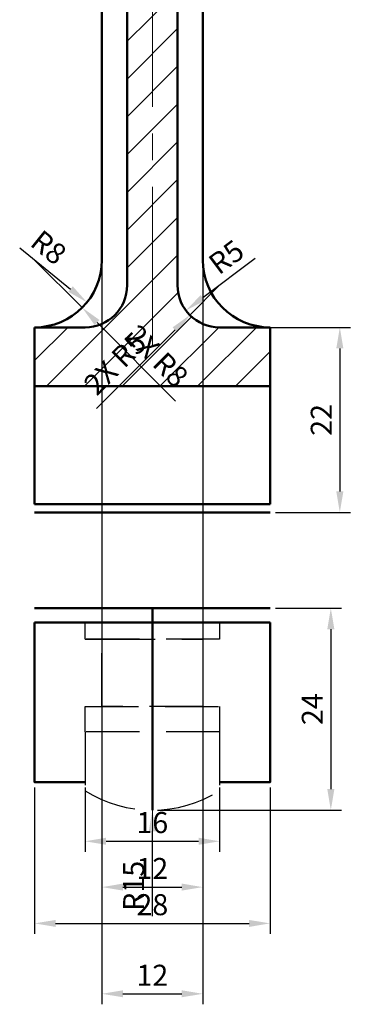
# Model space of a CAD drawing. Units: millimetres. Extents: x 2995 to 3180, y 2734 to 2968.
# Tile 2 of 3: x 3141 to 3180, y 2734 to 2851. Entities that reach past the tile are written whole.
import ezdxf

# ---------------------------------------------------------------- set-up
doc = ezdxf.new("R2010")
doc.units = ezdxf.units.MM
doc.linetypes.add('CENTER2', pattern=[28.575, 19.05, -3.175, 3.175, -3.175])
doc.linetypes.add('HIDDEN', pattern=[9.525, 6.35, -3.175])
for name, color, linetype, lineweight in [('M-CNTR', 1, 'CENTER2', 18), ('M-DIMS', 2, 'Continuous', 25), ('M-HATC', 8, 'Continuous', 18), ('M-HIDN', 4, 'HIDDEN', 25), ('M-OUTL', 7, 'Continuous', 50)]:
    doc.layers.add(name, color=color, linetype=linetype, lineweight=lineweight)
doc.styles.get("Standard").update_dxf_attribs({"font": 'arial.ttf'})
doc.dimstyles.new('ISO-25', dxfattribs={"dimtxt": 2.5, "dimasz": 2.5, "dimexe": 1.25, "dimexo": 0.625, "dimtad": 1, "dimtxsty": 'Standard', "dimcen": 2.5, "dimadec": 0, "dimazin": 0, "dimtfac": 1, "dimtmove": 0, "dimatfit": 3, "dimfxl": 1, "dimarcsym": 0})

# ---------------------------------------------------------------- blocks, each defined once
blk = doc.blocks.new('*D20')
at = {"layer": 'Defpoints', "color": 0, "transparency": 16777216}
for p in [(3170.35, 2814.6), (3170.93, 2792.6), (3179.23, 2792.6)]:
    blk.add_point(p, dxfattribs=at)
at = {"layer": 'M-DIMS', "color": 0, "lineweight": -2, "transparency": 16777216}
for p, q in [((3170.97, 2814.6), (3180.48, 2814.6)), ((3179.23, 2812.1), (3179.23, 2795.1)), ((3171.56, 2792.6), (3180.48, 2792.6))]:
    blk.add_line(p, q, dxfattribs=at)
at = {"layer": 'M-DIMS', "color": 0, "transparency": 16777216}
for points in [[(3178.81, 2812.1), (3179.65, 2812.1), (3179.23, 2814.6)], [(3178.81, 2795.1), (3179.65, 2795.1), (3179.23, 2792.6)]]:
    blk.add_solid(points, dxfattribs=at)
at = {"layer": 'M-DIMS', "color": 0, "transparency": 16777216, "insert": (3177.35, 2803.6), "char_height": 2.5, "attachment_point": 5, "rotation": 90}
blk.add_mtext('22', dxfattribs=at)
blk = doc.blocks.new('*D21')
at = {"layer": 'Defpoints', "color": 0, "transparency": 16777216}
for p in [(3170.93, 2781.22), (3156.93, 2757.22), (3178.16, 2757.22)]:
    blk.add_point(p, dxfattribs=at)
at = {"layer": 'M-DIMS', "color": 0, "lineweight": -2, "transparency": 16777216}
for p, q in [((3171.56, 2781.22), (3179.41, 2781.22)), ((3178.16, 2778.72), (3178.16, 2759.72)), ((3157.56, 2757.22), (3179.41, 2757.22))]:
    blk.add_line(p, q, dxfattribs=at)
at = {"layer": 'M-DIMS', "color": 0, "transparency": 16777216}
for points in [[(3177.74, 2778.72), (3178.58, 2778.72), (3178.16, 2781.22)], [(3177.74, 2759.72), (3178.58, 2759.72), (3178.16, 2757.22)]]:
    blk.add_solid(points, dxfattribs=at)
at = {"layer": 'M-DIMS', "color": 0, "transparency": 16777216, "insert": (3176.28, 2769.22), "char_height": 2.5, "attachment_point": 5, "rotation": 90}
blk.add_mtext('24', dxfattribs=at)
blk = doc.blocks.new('*D22')
at = {"layer": 'Defpoints', "color": 0, "transparency": 16777216}
for p in [(3148.93, 2760.53), (3164.93, 2760.53), (3164.93, 2753.52)]:
    blk.add_point(p, dxfattribs=at)
at = {"layer": 'M-DIMS', "color": 0, "lineweight": -2, "transparency": 16777216}
for p, q in [((3148.93, 2759.91), (3148.93, 2752.27)), ((3164.93, 2759.91), (3164.93, 2752.27)), ((3151.43, 2753.52), (3162.43, 2753.52))]:
    blk.add_line(p, q, dxfattribs=at)
at = {"layer": 'M-DIMS', "color": 0, "transparency": 16777216}
for points in [[(3151.43, 2753.94), (3151.43, 2753.1), (3148.93, 2753.52)], [(3162.43, 2753.94), (3162.43, 2753.1), (3164.93, 2753.52)]]:
    blk.add_solid(points, dxfattribs=at)
at = {"layer": 'M-DIMS', "color": 0, "transparency": 16777216, "insert": (3156.93, 2755.42), "char_height": 2.5, "attachment_point": 5}
blk.add_mtext('16', dxfattribs=at)
blk = doc.blocks.new('*D23')
at = {"layer": 'Defpoints', "color": 0, "transparency": 16777216}
for p in [(3150.93, 2769.53), (3162.93, 2769.53), (3162.93, 2748.07)]:
    blk.add_point(p, dxfattribs=at)
at = {"layer": 'M-DIMS', "color": 0, "lineweight": -2, "transparency": 16777216}
for p, q in [((3150.93, 2768.91), (3150.93, 2746.82)), ((3162.93, 2768.91), (3162.93, 2746.82)), ((3153.43, 2748.07), (3160.43, 2748.07))]:
    blk.add_line(p, q, dxfattribs=at)
at = {"layer": 'M-DIMS', "color": 0, "transparency": 16777216}
for points in [[(3153.43, 2748.49), (3153.43, 2747.66), (3150.93, 2748.07)], [(3160.43, 2748.49), (3160.43, 2747.66), (3162.93, 2748.07)]]:
    blk.add_solid(points, dxfattribs=at)
at = {"layer": 'M-DIMS', "color": 0, "transparency": 16777216, "insert": (3156.93, 2749.96), "char_height": 2.5, "attachment_point": 5}
blk.add_mtext('12', dxfattribs=at)
blk = doc.blocks.new('*D24')
at = {"layer": 'Defpoints', "color": 0, "transparency": 16777216}
for p in [(3142.93, 2760.53), (3170.93, 2760.53), (3170.93, 2743.76)]:
    blk.add_point(p, dxfattribs=at)
at = {"layer": 'M-DIMS', "color": 0, "lineweight": -2, "transparency": 16777216}
for p, q in [((3142.93, 2759.91), (3142.93, 2742.51)), ((3170.93, 2759.91), (3170.93, 2742.51)), ((3145.43, 2743.76), (3168.43, 2743.76))]:
    blk.add_line(p, q, dxfattribs=at)
at = {"layer": 'M-DIMS', "color": 0, "transparency": 16777216}
for points in [[(3145.43, 2744.17), (3145.43, 2743.34), (3142.93, 2743.76)], [(3168.43, 2744.17), (3168.43, 2743.34), (3170.93, 2743.76)]]:
    blk.add_solid(points, dxfattribs=at)
at = {"layer": 'M-DIMS', "color": 0, "transparency": 16777216, "insert": (3156.93, 2745.66), "char_height": 2.5, "attachment_point": 5}
blk.add_mtext('28', dxfattribs=at)
blk = doc.blocks.new('*D26')
at = {"layer": 'Defpoints', "color": 0, "transparency": 16777216}
for p in [(3164.93, 2819.6), (3160.92, 2816.61)]:
    blk.add_point(p, dxfattribs=at)
at = {"layer": 'M-DIMS', "color": 0, "lineweight": -2, "transparency": 16777216}
blk.add_line((3169.18, 2822.77), (3162.93, 2818.1), dxfattribs=at)
at = {"layer": 'M-DIMS', "color": 0, "transparency": 16777216}
blk.add_solid([(3162.68, 2818.43), (3163.18, 2817.77), (3160.92, 2816.61)], dxfattribs=at)
at = {"layer": 'M-DIMS', "color": 0, "transparency": 16777216, "insert": (3165.92, 2822.7), "char_height": 2.5, "attachment_point": 5, "rotation": 36.7449}
blk.add_mtext('R5', dxfattribs=at)
blk = doc.blocks.new('*D27')
at = {"layer": 'Defpoints', "color": 0, "transparency": 16777216}
for p in [(3142.93, 2822.6), (3149.16, 2817.57)]:
    blk.add_point(p, dxfattribs=at)
at = {"layer": 'M-DIMS', "color": 0, "lineweight": -2, "transparency": 16777216}
blk.add_line((3141.15, 2824.03), (3147.21, 2819.14), dxfattribs=at)
at = {"layer": 'M-DIMS', "color": 0, "transparency": 16777216}
blk.add_solid([(3147.47, 2819.47), (3146.95, 2818.82), (3149.16, 2817.57)], dxfattribs=at)
at = {"layer": 'M-DIMS', "color": 0, "transparency": 16777216, "insert": (3144.4, 2823.85), "char_height": 2.5, "attachment_point": 5, "rotation": 321.1153}
blk.add_mtext('R8', dxfattribs=at)
blk = doc.blocks.new('*D35')
at = {"layer": 'Defpoints', "color": 0, "transparency": 16777216}
for p in [(3150.93, 2916.6), (3162.93, 2916.6), (3162.93, 2735.39)]:
    blk.add_point(p, dxfattribs=at)
at = {"layer": 'M-DIMS', "color": 0, "lineweight": -2, "transparency": 16777216}
for p, q in [((3150.93, 2915.97), (3150.93, 2734.14)), ((3162.93, 2915.97), (3162.93, 2734.14)), ((3153.43, 2735.39), (3160.43, 2735.39))]:
    blk.add_line(p, q, dxfattribs=at)
at = {"layer": 'M-DIMS', "color": 0, "transparency": 16777216}
for points in [[(3153.43, 2735.81), (3153.43, 2734.98), (3150.93, 2735.39)], [(3160.43, 2735.81), (3160.43, 2734.98), (3162.93, 2735.39)]]:
    blk.add_solid(points, dxfattribs=at)
at = {"layer": 'M-DIMS', "color": 0, "transparency": 16777216, "insert": (3156.93, 2737.27), "char_height": 2.5, "attachment_point": 5}
blk.add_mtext('12', dxfattribs=at)
blk = doc.blocks.new('*D54')
at = {"layer": 'Defpoints', "color": 0, "transparency": 16777216}
for p in [(3142.93, 2822.6), (3148.59, 2816.94)]:
    blk.add_point(p, dxfattribs=at)
at = {"layer": 'M-DIMS', "color": 0, "lineweight": -2, "transparency": 16777216}
for p, q in [((3142.93, 2822.6), (3148.59, 2816.94)), ((3159.69, 2805.84), (3150.36, 2815.17))]:
    blk.add_line(p, q, dxfattribs=at)
at = {"layer": 'M-DIMS', "color": 0, "transparency": 16777216}
blk.add_solid([(3150.65, 2815.47), (3150.06, 2814.88), (3148.59, 2816.94)], dxfattribs=at)
at = {"layer": 'M-DIMS', "color": 0, "transparency": 16777216, "insert": (3157.25, 2810.97), "char_height": 2.5, "attachment_point": 5, "rotation": 315.0011}
blk.add_mtext('2X R8', dxfattribs=at)
blk = doc.blocks.new('*D55')
at = {"layer": 'Defpoints', "color": 0, "transparency": 16777216}
for p in [(3164.93, 2819.6), (3161.39, 2816.06)]:
    blk.add_point(p, dxfattribs=at)
at = {"layer": 'M-DIMS', "color": 0, "lineweight": -2, "transparency": 16777216}
for p, q in [((3164.93, 2819.6), (3161.39, 2816.06)), ((3150.28, 2804.95), (3159.63, 2814.29))]:
    blk.add_line(p, q, dxfattribs=at)
at = {"layer": 'M-DIMS', "color": 0, "transparency": 16777216}
blk.add_solid([(3159.33, 2814.59), (3159.92, 2814), (3161.39, 2816.06)], dxfattribs=at)
at = {"layer": 'M-DIMS', "color": 0, "transparency": 16777216, "insert": (3152.73, 2810.08), "char_height": 2.5, "attachment_point": 5, "rotation": 45}
blk.add_mtext('2X R5', dxfattribs=at)
blk = doc.blocks.new('*D56')
at = {"layer": 'Defpoints', "color": 0, "transparency": 16777216}
for p in [(3156.93, 2772.22), (3156.93, 2757.22)]:
    blk.add_point(p, dxfattribs=at)
at = {"layer": 'M-DIMS', "color": 0, "lineweight": -2, "transparency": 16777216}
for p, q in [((3156.93, 2772.22), (3156.93, 2757.22)), ((3156.93, 2744.6), (3156.93, 2754.72))]:
    blk.add_line(p, q, dxfattribs=at)
at = {"layer": 'M-DIMS', "color": 0, "transparency": 16777216}
blk.add_solid([(3156.51, 2754.72), (3157.35, 2754.72), (3156.93, 2757.22)], dxfattribs=at)
at = {"layer": 'M-DIMS', "color": 0, "transparency": 16777216, "insert": (3155.03, 2748.22), "char_height": 2.5, "attachment_point": 5, "rotation": 89.9985}
blk.add_mtext('R15', dxfattribs=at)

msp = doc.modelspace()

# ---------------------------------------------------------------- hatches: boundary and pattern name
at = {"layer": 'M-HATC'}
h = msp.add_hatch(dxfattribs=at)
h.set_pattern_fill('ANSI31', color=256)
h.paths.add_polyline_path([(3147.9304, 2924.5964), (3147.9304, 2921.5964, -0.36997107), (3153.9304, 2916.5964), (3153.9304, 2819.5964, -0.41421356), (3148.9304, 2814.5964), (3142.9304, 2814.5964), (3142.9304, 2807.5964), (3170.9304, 2807.5964), (3170.9304, 2814.5964), (3164.9304, 2814.5964, -0.41421356), (3159.9304, 2819.5964), (3159.9304, 2916.5964, -0.36997107), (3165.9304, 2921.5964), (3165.9304, 2924.5964)])

# ---------------------------------------------------------------- linework, layer by layer
at = {"layer": 'M-CNTR'}
for p, q in [((3156.9304, 2945.5964), (3156.9304, 2810.5964)), ((3156.9304, 2779.5315), (3156.9304, 2746.2676))]:
    msp.add_line(p, q, dxfattribs=at)
at = {"layer": 'M-HIDN'}
for p, q in [((3148.9304, 2777.5315), (3150.9304, 2777.5315)), ((3148.9304, 2766.5315), (3148.9304, 2759.5315)), ((3164.9304, 2766.5315), (3164.9304, 2759.5315))]:
    msp.add_line(p, q, dxfattribs=at)
for points in [[(3148.9304, 2781.2201), (3164.9304, 2781.2201)], [(3164.9304, 2779.5315), (3164.9304, 2777.5315), (3148.9304, 2777.5315), (3148.9304, 2779.5315)]]:
    msp.add_lwpolyline(points, dxfattribs=at)
for points in [[(3150.9304, 2777.5315), (3162.9304, 2777.5315), (3162.9304, 2769.5315), (3150.9304, 2769.5315)], [(3148.9304, 2769.5315), (3164.9304, 2769.5315), (3164.9304, 2766.5315), (3148.9304, 2766.5315)]]:
    msp.add_lwpolyline(points, close=True, dxfattribs=at)
msp.add_arc((3156.9304, 2772.2201), 15, 237.769047, 302.230953, dxfattribs=at)
at = {"layer": 'M-OUTL'}
for p, q in [((3150.9304, 2822.5964), (3150.9304, 2916.5964)), ((3153.9304, 2916.5964), (3153.9304, 2819.5964)), ((3159.9304, 2916.5964), (3159.9304, 2819.5964)), ((3162.9304, 2916.5964), (3162.9304, 2822.5964)), ((3142.9304, 2807.5964), (3142.9304, 2814.5964)), ((3142.9304, 2814.5964), (3148.9304, 2814.5964)), ((3142.9304, 2814.5964), (3142.9304, 2814.5964)), ((3164.9304, 2814.5964), (3170.9304, 2814.5964)), ((3170.9304, 2814.5964), (3170.9304, 2807.5964)), ((3170.9304, 2814.5964), (3170.9304, 2814.5964)), ((3170.9304, 2814.5964), (3170.9304, 2793.5964)), ((3170.9304, 2807.5964), (3142.9304, 2807.5964)), ((3142.9304, 2793.5964), (3142.9304, 2807.5964)), ((3142.9304, 2793.5964), (3170.9304, 2793.5964)), ((3170.9304, 2792.5964), (3142.9304, 2792.5964)), ((3156.9304, 2757.2201), (3156.9304, 2781.2201)), ((3142.9304, 2779.5315), (3170.9304, 2779.5315))]:
    msp.add_line(p, q, dxfattribs=at)
for points in [[(3142.9304, 2781.2201), (3170.9304, 2781.2201)], [(3148.9304, 2760.5315), (3142.9304, 2760.5315), (3142.9304, 2779.5315)], [(3170.9304, 2779.5315), (3170.9304, 2760.5315), (3164.9304, 2760.5315)]]:
    msp.add_lwpolyline(points, dxfattribs=at)
for centre, radius, start, end in [((3142.9304, 2822.5964), 8, 270, 360), ((3170.9304, 2822.5964), 8, 180, 270), ((3148.9304, 2819.5964), 5, 270, 0), ((3164.9304, 2819.5964), 5, 180, 270)]:
    msp.add_arc(centre, radius, start, end, dxfattribs=at)

# ---------------------------------------------------------------- dimensions: what is measured, and where the dimension line sits
at = {"layer": 'M-DIMS'}
for base, p1, p2, override, picture, middle in [((3162.9304, 2735.3926), (3150.9304, 2916.5964), (3162.9304, 2916.5964), {"dimdec": 0, "dimlfac": 1, "dimrnd": 0, "dimzin": 0, "dimdsep": 46, "dimlunit": 2}, '*D35', (3156.9304, 2737.2727)), ((3162.9304, 2748.0749), (3150.9304, 2769.5315), (3162.9304, 2769.5315), {"dimclrd": 0, "dimclre": 0, "dimclrt": 0}, '*D23', (3156.9304, 2749.9551)), ((3170.9304, 2743.7569), (3142.9304, 2760.5315), (3170.9304, 2760.5315), {"dimclrd": 0, "dimclre": 0, "dimclrt": 0}, '*D24', (3156.9304, 2745.6584)), ((3164.9304, 2753.5194), (3148.9304, 2760.5315), (3164.9304, 2760.5315), {"dimclrd": 0, "dimclre": 0, "dimclrt": 0}, '*D22', (3156.9304, 2755.4208))]:
    dim = msp.add_linear_dim(base=base, p1=p1, p2=p2, dimstyle='ISO-25', override=override, dxfattribs=at)
    dim.commit()
    dim.dimension.update_dxf_attribs({"geometry": picture, "text_midpoint": middle})
for center, mpoint, override, picture, middle in [((3142.9304, 2822.5964), (3149.1577, 2817.5743), {"dimclrd": 0, "dimclre": 0, "dimclrt": 0}, '*D27', (3143.2081, 2822.3724)), ((3164.9304, 2819.5964), (3160.9239, 2816.6051), {"dimclrd": 0, "dimclre": 0, "dimclrt": 0}, '*D26', (3167.0539, 2821.1818)), ((3156.9304, 2772.2201), (3156.93, 2757.2201), {"dimdec": 0, "dimlfac": 1, "dimrnd": 0, "dimzin": 0, "dimdsep": 46, "dimlunit": 2}, '*D56', (3156.9298, 2748.2201))]:
    dim = msp.add_radius_dim(center=center, mpoint=mpoint, dimstyle='ISO-25', override=override, dxfattribs=at)
    dim.commit()
    dim.dimension.update_dxf_attribs({"geometry": picture, "text_midpoint": middle, "dimtype": 164})
for center, mpoint, picture, middle in [((3142.9304, 2822.5964), (3148.5874, 2816.9396), '*D54', (3157.2509, 2810.9655)), ((3164.9304, 2819.5964), (3161.3949, 2816.0609), '*D55', (3152.7266, 2810.0817))]:
    dim = msp.add_radius_dim(center=center, mpoint=mpoint, text='2X <>', dimstyle='ISO-25', override={"dimdec": 0, "dimlfac": 1, "dimrnd": 0, "dimzin": 0, "dimdsep": 46, "dimlunit": 2}, dxfattribs=at)
    dim.commit()
    dim.dimension.update_dxf_attribs({"geometry": picture, "text_midpoint": middle})
for base, p1, p2, picture, middle in [((3179.2283, 2792.5964), (3170.3461, 2814.5964), (3170.9304, 2792.5964), '*D20', (3177.3482, 2803.5964)), ((3178.16, 2757.2201), (3170.9304, 2781.2201), (3156.9304, 2757.2201), '*D21', (3176.2799, 2769.2201))]:
    dim = msp.add_linear_dim(base=base, p1=p1, p2=p2, angle=90, dimstyle='ISO-25', override={"dimclrd": 0, "dimclre": 0, "dimclrt": 0}, dxfattribs=at)
    dim.commit()
    dim.dimension.update_dxf_attribs({"geometry": picture, "text_midpoint": middle})

doc.saveas('drawing.dxf')
